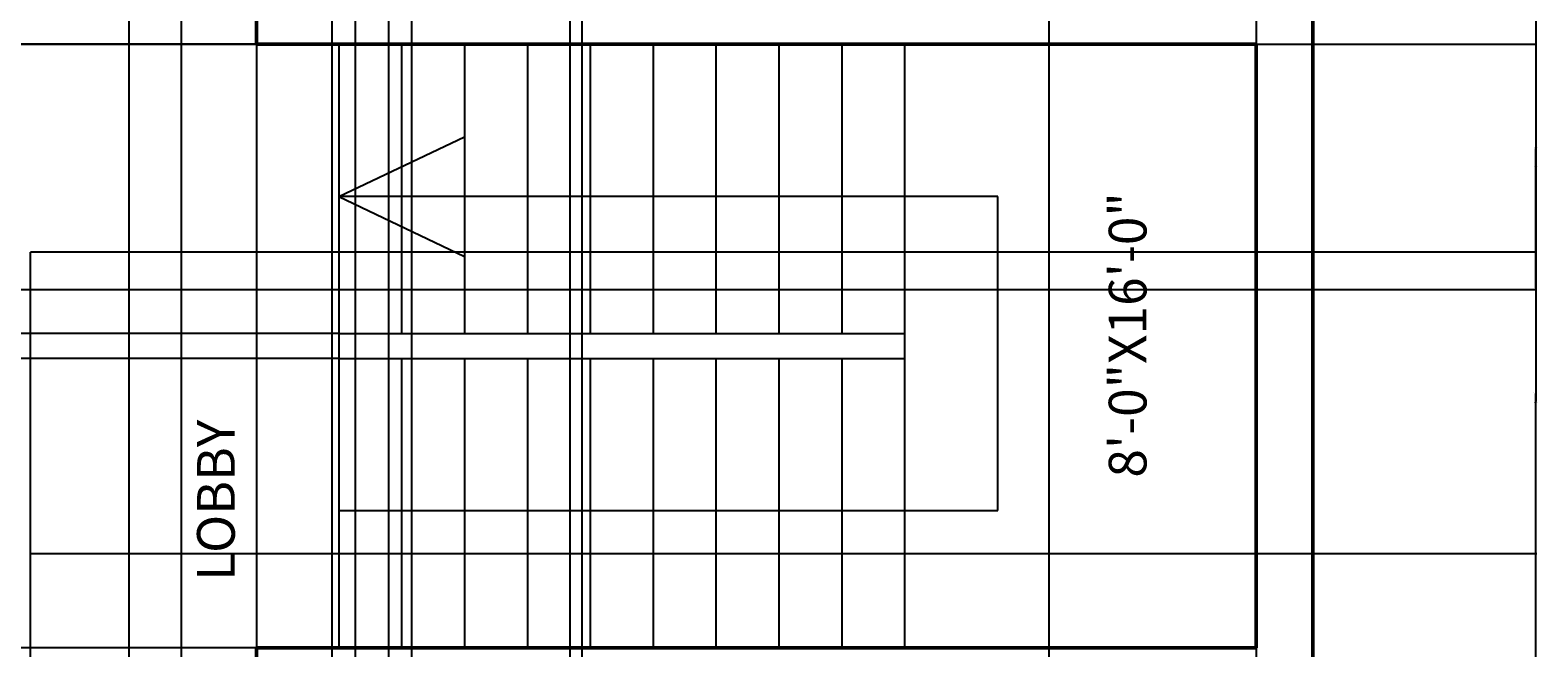
# Model space of a CAD drawing. Units: inches. Extents: x 3 to 576, y -689 to 51.
# Tile 13 of 21: x 336 to 576, y -359 to -261. Entities that reach past the tile are written whole.
import ezdxf

# ---------------------------------------------------------------- set-up
doc = ezdxf.new("R2010")
doc.units = ezdxf.units.IN
doc.header["$MEASUREMENT"] = 0
for name, color, linetype, lineweight in [('A-ANNO-DIMS', 2, 'Continuous', 18), ('A-AREA-IDEN', 7, 'Continuous', 18), ('A-FLOR-STRS', 7, 'Continuous', 25), ('A-WALL', 7, 'Continuous', 50)]:
    doc.layers.add(name, color=color, linetype=linetype, lineweight=lineweight)
doc.styles.get("Standard").update_dxf_attribs({"font": 'arial.ttf'})
doc.dimstyles.get("Standard").update_dxf_attribs({"dimtxt": 0.18, "dimasz": 0.18, "dimexe": 0.18, "dimexo": 0.0625, "dimgap": 0.09, "dimtad": 0, "dimtih": 1, "dimtoh": 1, "dimdec": 0, "dimzin": 0, "dimdsep": 46, "dimlunit": 3, "dimtxsty": 'Standard', "dimcen": 0.09, "dimadec": 0, "dimazin": 0, "dimtfac": 1, "dimtdec": 0, "dimtofl": 0, "dimtmove": 0, "dimatfit": 3, "dimfxl": 1, "dimtolj": 1, "dimtzin": 0, "dimarcsym": 0})

# ---------------------------------------------------------------- blocks, each defined once
blk = doc.blocks.new('*D39')
at = {"layer": 'A-ANNO-DIMS', "color": 0, "lineweight": -2, "transparency": 16777216}
for p, q in [((540.36, 15.69), (575.92, 15.69)), ((575.74, 15.51), (575.74, -318.63)), ((575.74, -653.13), (575.74, -318.99)), ((540.36, -653.31), (575.92, -653.31))]:
    blk.add_line(p, q, dxfattribs=at)
at = {"layer": 'A-ANNO-DIMS', "color": 0, "transparency": 16777216}
for points in [[(575.71, 15.51), (575.77, 15.51), (575.74, 15.69)], [(575.71, -653.13), (575.77, -653.13), (575.74, -653.31)]]:
    blk.add_solid(points, dxfattribs=at)
at = {"layer": 'Defpoints', "color": 0, "transparency": 16777216}
for p in [(540.29, 15.69), (540.29, -653.31), (575.74, -653.31)]:
    blk.add_point(p, dxfattribs=at)
at = {"layer": 'A-ANNO-DIMS', "color": 0, "transparency": 16777216, "insert": (575.74, -318.81), "char_height": 0.18, "attachment_point": 5}
blk.add_mtext('\\A1;55\'-9"', dxfattribs=at)
blk = doc.blocks.new('*D63')
at = {"layer": 'A-ANNO-DIMS', "color": 0, "lineweight": -2, "transparency": 16777216}
for p, q in [((47.36, -263.31), (575.92, -263.31)), ((575.74, -263.49), (575.74, -282.63)), ((575.74, -302.13), (575.74, -282.99)), ((47.36, -302.31), (575.92, -302.31))]:
    blk.add_line(p, q, dxfattribs=at)
at = {"layer": 'A-ANNO-DIMS', "color": 0, "transparency": 16777216}
for points in [[(575.71, -263.49), (575.77, -263.49), (575.74, -263.31)], [(575.71, -302.13), (575.77, -302.13), (575.74, -302.31)]]:
    blk.add_solid(points, dxfattribs=at)
at = {"layer": 'Defpoints', "color": 0, "transparency": 16777216}
for p in [(47.29, -263.31), (47.29, -302.31), (575.74, -302.31)]:
    blk.add_point(p, dxfattribs=at)
at = {"layer": 'A-ANNO-DIMS', "color": 0, "transparency": 16777216, "insert": (575.74, -282.81), "char_height": 0.18, "attachment_point": 5}
blk.add_mtext('\\A1;3\'-3"', dxfattribs=at)
blk = doc.blocks.new('*D68')
at = {"layer": 'A-ANNO-DIMS', "color": 0, "lineweight": -2, "transparency": 16777216}
for p, q in [((531.23, -254.31), (2.66, -254.31)), ((2.84, -254.49), (2.84, -258.63)), ((2.84, -263.13), (2.84, -258.99)), ((531.23, -263.31), (2.66, -263.31))]:
    blk.add_line(p, q, dxfattribs=at)
at = {"layer": 'A-ANNO-DIMS', "color": 0, "transparency": 16777216}
for points in [[(2.81, -254.49), (2.87, -254.49), (2.84, -254.31)], [(2.81, -263.13), (2.87, -263.13), (2.84, -263.31)]]:
    blk.add_solid(points, dxfattribs=at)
at = {"layer": 'Defpoints', "color": 0, "transparency": 16777216}
for p in [(531.29, -254.31), (2.84, -263.31), (531.29, -263.31)]:
    blk.add_point(p, dxfattribs=at)
at = {"layer": 'A-ANNO-DIMS', "color": 0, "transparency": 16777216, "insert": (2.84, -258.81), "char_height": 0.18, "attachment_point": 5}
blk.add_mtext('\\A1;0\'-9"', dxfattribs=at)
blk = doc.blocks.new('*D69')
at = {"layer": 'A-ANNO-DIMS', "color": 0, "lineweight": -2, "transparency": 16777216}
for p, q in [((531.23, -263.31), (2.66, -263.31)), ((2.84, -263.49), (2.84, -311.13)), ((2.84, -359.13), (2.84, -311.49)), ((531.23, -359.31), (2.66, -359.31))]:
    blk.add_line(p, q, dxfattribs=at)
at = {"layer": 'A-ANNO-DIMS', "color": 0, "transparency": 16777216}
for points in [[(2.81, -263.49), (2.87, -263.49), (2.84, -263.31)], [(2.81, -359.13), (2.87, -359.13), (2.84, -359.31)]]:
    blk.add_solid(points, dxfattribs=at)
at = {"layer": 'Defpoints', "color": 0, "transparency": 16777216}
for p in [(531.29, -263.31), (2.84, -359.31), (531.29, -359.31)]:
    blk.add_point(p, dxfattribs=at)
at = {"layer": 'A-ANNO-DIMS', "color": 0, "transparency": 16777216, "insert": (2.84, -311.31), "char_height": 0.18, "attachment_point": 5}
blk.add_mtext('\\A1;8\'-0"', dxfattribs=at)
blk = doc.blocks.new('*D76')
at = {"layer": 'A-ANNO-DIMS', "color": 0, "lineweight": -2, "transparency": 16777216}
for p, q in [((372.29, -263.37), (372.29, -688.94)), ((336.29, -296.37), (336.29, -688.94)), ((336.47, -688.76), (353.96, -688.76)), ((372.11, -688.76), (354.62, -688.76))]:
    blk.add_line(p, q, dxfattribs=at)
at = {"layer": 'A-ANNO-DIMS', "color": 0, "transparency": 16777216}
for points in [[(336.47, -688.73), (336.47, -688.79), (336.29, -688.76)], [(372.11, -688.73), (372.11, -688.79), (372.29, -688.76)]]:
    blk.add_solid(points, dxfattribs=at)
at = {"layer": 'Defpoints', "color": 0, "transparency": 16777216}
for p in [(372.29, -263.31), (336.29, -296.31), (372.29, -688.76)]:
    blk.add_point(p, dxfattribs=at)
at = {"layer": 'A-ANNO-DIMS', "color": 0, "transparency": 16777216, "insert": (354.29, -688.76), "char_height": 0.18, "attachment_point": 5}
blk.add_mtext('\\A1;3\'-0"', dxfattribs=at)
blk = doc.blocks.new('*D77')
at = {"layer": 'A-ANNO-DIMS', "color": 0, "lineweight": -2, "transparency": 16777216}
for p, q in [((372.29, -263.37), (372.29, -688.94)), ((531.29, -263.37), (531.29, -688.94)), ((372.47, -688.76), (451.4, -688.76)), ((531.11, -688.76), (452.18, -688.76))]:
    blk.add_line(p, q, dxfattribs=at)
at = {"layer": 'A-ANNO-DIMS', "color": 0, "transparency": 16777216}
for points in [[(372.47, -688.73), (372.47, -688.79), (372.29, -688.76)], [(531.11, -688.73), (531.11, -688.79), (531.29, -688.76)]]:
    blk.add_solid(points, dxfattribs=at)
at = {"layer": 'Defpoints', "color": 0, "transparency": 16777216}
for p in [(372.29, -263.31), (531.29, -263.31), (531.29, -688.76)]:
    blk.add_point(p, dxfattribs=at)
at = {"layer": 'A-ANNO-DIMS', "color": 0, "transparency": 16777216, "insert": (451.79, -688.76), "char_height": 0.18, "attachment_point": 5}
blk.add_mtext('\\A1;13\'-3"', dxfattribs=at)
blk = doc.blocks.new('*D78')
at = {"layer": 'A-ANNO-DIMS', "color": 0, "lineweight": -2, "transparency": 16777216}
for p, q in [((336.36, -263.31), (575.92, -263.31)), ((575.74, -263.49), (575.74, -279.63)), ((575.74, -296.13), (575.74, -279.99)), ((336.36, -296.31), (575.92, -296.31))]:
    blk.add_line(p, q, dxfattribs=at)
at = {"layer": 'A-ANNO-DIMS', "color": 0, "transparency": 16777216}
for points in [[(575.71, -263.49), (575.77, -263.49), (575.74, -263.31)], [(575.71, -296.13), (575.77, -296.13), (575.74, -296.31)]]:
    blk.add_solid(points, dxfattribs=at)
at = {"layer": 'Defpoints', "color": 0, "transparency": 16777216}
for p in [(336.29, -263.31), (336.29, -296.31), (575.74, -296.31)]:
    blk.add_point(p, dxfattribs=at)
at = {"layer": 'A-ANNO-DIMS', "color": 0, "transparency": 16777216, "insert": (575.74, -279.81), "char_height": 0.18, "attachment_point": 5}
blk.add_mtext('\\A1;2\'-9"', dxfattribs=at)
blk = doc.blocks.new('*D79')
at = {"layer": 'A-ANNO-DIMS', "color": 0, "lineweight": -2, "transparency": 16777216}
for p, q in [((336.36, -296.31), (575.92, -296.31)), ((575.74, -296.49), (575.74, -320.13)), ((575.74, -344.13), (575.74, -320.49)), ((336.36, -344.31), (575.92, -344.31))]:
    blk.add_line(p, q, dxfattribs=at)
at = {"layer": 'A-ANNO-DIMS', "color": 0, "transparency": 16777216}
for points in [[(575.71, -296.49), (575.77, -296.49), (575.74, -296.31)], [(575.71, -344.13), (575.77, -344.13), (575.74, -344.31)]]:
    blk.add_solid(points, dxfattribs=at)
at = {"layer": 'Defpoints', "color": 0, "transparency": 16777216}
for p in [(336.29, -296.31), (336.29, -344.31), (575.74, -344.31)]:
    blk.add_point(p, dxfattribs=at)
at = {"layer": 'A-ANNO-DIMS', "color": 0, "transparency": 16777216, "insert": (575.74, -320.31), "char_height": 0.18, "attachment_point": 5}
blk.add_mtext('\\A1;4\'-0"', dxfattribs=at)
blk = doc.blocks.new('*D84')
at = {"layer": 'A-ANNO-DIMS', "color": 0, "lineweight": -2, "transparency": 16777216}
for p, q in [((385.3, -263.31), (2.66, -263.31)), ((2.84, -263.49), (2.84, -286.13)), ((2.84, -309.13), (2.84, -286.49)), ((385.3, -309.31), (2.66, -309.31))]:
    blk.add_line(p, q, dxfattribs=at)
at = {"layer": 'A-ANNO-DIMS', "color": 0, "transparency": 16777216}
for points in [[(2.81, -263.49), (2.87, -263.49), (2.84, -263.31)], [(2.81, -309.13), (2.87, -309.13), (2.84, -309.31)]]:
    blk.add_solid(points, dxfattribs=at)
at = {"layer": 'Defpoints', "color": 0, "transparency": 16777216}
for p in [(385.37, -263.31), (2.84, -309.31), (385.37, -309.31)]:
    blk.add_point(p, dxfattribs=at)
at = {"layer": 'A-ANNO-DIMS', "color": 0, "transparency": 16777216, "insert": (2.84, -286.31), "char_height": 0.18, "attachment_point": 5}
blk.add_mtext('\\A1;3\'-10"', dxfattribs=at)
blk = doc.blocks.new('*D85')
at = {"layer": 'A-ANNO-DIMS', "color": 0, "lineweight": -2, "transparency": 16777216}
for p, q in [((385.3, -313.31), (2.66, -313.31)), ((2.84, -313.49), (2.84, -336.13)), ((2.84, -359.13), (2.84, -336.49)), ((385.3, -359.31), (2.66, -359.31))]:
    blk.add_line(p, q, dxfattribs=at)
at = {"layer": 'A-ANNO-DIMS', "color": 0, "transparency": 16777216}
for points in [[(2.81, -313.49), (2.87, -313.49), (2.84, -313.31)], [(2.81, -359.13), (2.87, -359.13), (2.84, -359.31)]]:
    blk.add_solid(points, dxfattribs=at)
at = {"layer": 'Defpoints', "color": 0, "transparency": 16777216}
for p in [(385.37, -313.31), (2.84, -359.31), (385.37, -359.31)]:
    blk.add_point(p, dxfattribs=at)
at = {"layer": 'A-ANNO-DIMS', "color": 0, "transparency": 16777216, "insert": (2.84, -336.31), "char_height": 0.18, "attachment_point": 5}
blk.add_mtext('\\A1;3\'-10"', dxfattribs=at)
blk = doc.blocks.new('*D94')
at = {"layer": 'A-ANNO-DIMS', "color": 0, "lineweight": -2, "transparency": 16777216}
for p, q in [((393.29, -136.9), (393.29, -688.94)), ((422.14, -136.9), (422.14, -688.94)), ((393.47, -688.76), (407.39, -688.76)), ((421.96, -688.76), (408.05, -688.76))]:
    blk.add_line(p, q, dxfattribs=at)
at = {"layer": 'A-ANNO-DIMS', "color": 0, "transparency": 16777216}
for points in [[(393.47, -688.73), (393.47, -688.79), (393.29, -688.76)], [(421.96, -688.73), (421.96, -688.79), (422.14, -688.76)]]:
    blk.add_solid(points, dxfattribs=at)
at = {"layer": 'Defpoints', "color": 0, "transparency": 16777216}
for p in [(393.29, -136.84), (422.14, -136.84), (422.14, -688.76)]:
    blk.add_point(p, dxfattribs=at)
at = {"layer": 'A-ANNO-DIMS', "color": 0, "transparency": 16777216, "insert": (407.72, -688.76), "char_height": 0.18, "attachment_point": 5}
blk.add_mtext('\\A1;2\'-5"', dxfattribs=at)
blk = doc.blocks.new('*D96')
at = {"layer": 'A-ANNO-DIMS', "color": 0, "lineweight": -2, "transparency": 16777216}
for p, q in [((397.02, -506.04), (397.02, 51.32)), ((397.2, 51.14), (410.22, 51.14)), ((423.91, 51.14), (410.89, 51.14)), ((424.09, -506.04), (424.09, 51.32))]:
    blk.add_line(p, q, dxfattribs=at)
at = {"layer": 'A-ANNO-DIMS', "color": 0, "transparency": 16777216}
for points in [[(397.2, 51.17), (397.2, 51.11), (397.02, 51.14)], [(423.91, 51.17), (423.91, 51.11), (424.09, 51.14)]]:
    blk.add_solid(points, dxfattribs=at)
at = {"layer": 'Defpoints', "color": 0, "transparency": 16777216}
for p in [(424.09, 51.14), (397.02, -506.1), (424.09, -506.1)]:
    blk.add_point(p, dxfattribs=at)
at = {"layer": 'A-ANNO-DIMS', "color": 0, "transparency": 16777216, "insert": (410.56, 51.14), "char_height": 0.18, "attachment_point": 5}
blk.add_mtext('\\A1;2\'-3"', dxfattribs=at)
blk = doc.blocks.new('*D103')
at = {"layer": 'A-ANNO-DIMS', "color": 0, "lineweight": -2, "transparency": 16777216}
for p, q in [((498.29, -50.37), (498.29, -688.94)), ((531.29, -50.37), (531.29, -688.94)), ((498.47, -688.76), (514.46, -688.76)), ((531.11, -688.76), (515.12, -688.76))]:
    blk.add_line(p, q, dxfattribs=at)
at = {"layer": 'A-ANNO-DIMS', "color": 0, "transparency": 16777216}
for points in [[(498.47, -688.73), (498.47, -688.79), (498.29, -688.76)], [(531.11, -688.73), (531.11, -688.79), (531.29, -688.76)]]:
    blk.add_solid(points, dxfattribs=at)
at = {"layer": 'Defpoints', "color": 0, "transparency": 16777216}
for p in [(498.29, -50.31), (531.29, -50.31), (531.29, -688.76)]:
    blk.add_point(p, dxfattribs=at)
at = {"layer": 'A-ANNO-DIMS', "color": 0, "transparency": 16777216, "insert": (514.79, -688.76), "char_height": 0.18, "attachment_point": 5}
blk.add_mtext('\\A1;2\'-9"', dxfattribs=at)
blk = doc.blocks.new('*D116')
at = {"layer": 'A-ANNO-DIMS', "color": 0, "lineweight": -2, "transparency": 16777216}
for p, q in [((360.29, -134.37), (360.29, -688.94)), ((384.29, -134.37), (384.29, -688.94)), ((360.47, -688.76), (371.96, -688.76)), ((384.11, -688.76), (372.62, -688.76))]:
    blk.add_line(p, q, dxfattribs=at)
at = {"layer": 'A-ANNO-DIMS', "color": 0, "transparency": 16777216}
for points in [[(360.47, -688.73), (360.47, -688.79), (360.29, -688.76)], [(384.11, -688.73), (384.11, -688.79), (384.29, -688.76)]]:
    blk.add_solid(points, dxfattribs=at)
at = {"layer": 'Defpoints', "color": 0, "transparency": 16777216}
for p in [(360.29, -134.31), (384.29, -134.31), (384.29, -688.76)]:
    blk.add_point(p, dxfattribs=at)
at = {"layer": 'A-ANNO-DIMS', "color": 0, "transparency": 16777216, "insert": (372.29, -688.76), "char_height": 0.18, "attachment_point": 5}
blk.add_mtext('\\A1;2\'-0"', dxfattribs=at)
blk = doc.blocks.new('*D118')
at = {"layer": 'A-ANNO-DIMS', "color": 0, "lineweight": -2, "transparency": 16777216}
for p, q in [((352.02, -506.25), (352.02, 51.32)), ((352.2, 51.14), (369.69, 51.14)), ((387.84, 51.14), (370.35, 51.14)), ((388.02, -506.25), (388.02, 51.32))]:
    blk.add_line(p, q, dxfattribs=at)
at = {"layer": 'A-ANNO-DIMS', "color": 0, "transparency": 16777216}
for points in [[(352.2, 51.17), (352.2, 51.11), (352.02, 51.14)], [(387.84, 51.17), (387.84, 51.11), (388.02, 51.14)]]:
    blk.add_solid(points, dxfattribs=at)
at = {"layer": 'Defpoints', "color": 0, "transparency": 16777216}
for p in [(388.02, 51.14), (352.02, -506.31), (388.02, -506.31)]:
    blk.add_point(p, dxfattribs=at)
at = {"layer": 'A-ANNO-DIMS', "color": 0, "transparency": 16777216, "insert": (370.02, 51.14), "char_height": 0.18, "attachment_point": 5}
blk.add_mtext('\\A1;3\'-0"', dxfattribs=at)

msp = doc.modelspace()

# ---------------------------------------------------------------- linework, layer by layer
at = {"layer": 'A-FLOR-STRS'}
for p, q in [((385.37, -263.31), (385.37, -359.31)), ((395.37, -263.31), (395.37, -309.31)), ((405.37, -263.31), (405.37, -309.31)), ((415.37, -263.31), (415.37, -309.31)), ((425.37, -263.31), (425.37, -309.31)), ((435.37, -263.31), (435.37, -309.31)), ((445.37, -263.31), (445.37, -309.31)), ((455.37, -263.31), (455.37, -309.31)), ((465.37, -263.31), (465.37, -309.31)), ((475.37, -263.31), (475.37, -359.31)), ((385.37, -287.55), (405.37, -278.02)), ((490.22, -287.55), (385.37, -287.55)), ((385.37, -287.55), (405.37, -297.09)), ((490.22, -337.45), (490.22, -287.55)), ((385.37, -309.31), (475.37, -309.31)), ((385.37, -313.31), (475.37, -313.31)), ((395.37, -313.31), (395.37, -359.31)), ((405.37, -313.31), (405.37, -359.31)), ((415.37, -313.31), (415.37, -359.31)), ((425.37, -313.31), (425.37, -359.31)), ((435.37, -313.31), (435.37, -359.31)), ((445.37, -313.31), (445.37, -359.31)), ((455.37, -313.31), (455.37, -359.31)), ((465.37, -313.31), (465.37, -359.31)), ((385.37, -337.45), (490.22, -337.45))]:
    msp.add_line(p, q, dxfattribs=at)
at = {"layer": 'A-WALL'}
for p, q in [((540.29, 15.69), (540.29, -653.31)), ((372.29, -254.31), (372.29, -263.31)), ((372.29, -263.31), (531.29, -263.31)), ((531.29, -263.31), (531.29, -359.31)), ((372.29, -359.31), (531.29, -359.31)), ((372.29, -368.31), (372.29, -359.31))]:
    msp.add_line(p, q, dxfattribs=at)

# ---------------------------------------------------------------- texts
at = {"layer": 'A-AREA-IDEN', "insert": (507.84, -332.24), "char_height": 6, "attachment_point": 1, "rotation": 90}
msp.add_mtext_dynamic_manual_height_columns('8\'-0"X16\'-0"', width=6, gutter_width=1, heights=[0], dxfattribs=at)
at = {"layer": 'A-AREA-IDEN', "insert": (362.84, -348.66), "char_height": 6, "attachment_point": 1, "rotation": 90}
msp.add_mtext('LOBBY', dxfattribs=at)

# ---------------------------------------------------------------- dimensions: what is measured, and where the dimension line sits
at = {"layer": 'A-ANNO-DIMS'}
for base, p1, p2, picture, middle in [((388.02, 51.14), (352.02, -506.31), (388.02, -506.31), '*D118', (370.02, 51.14)), ((424.09, 51.14), (397.02, -506.1), (424.09, -506.1), '*D96', (410.56, 51.14)), ((531.29, -688.76), (498.29, -50.31), (531.29, -50.31), '*D103', (514.79, -688.76)), ((384.29, -688.76), (360.29, -134.31), (384.29, -134.31), '*D116', (372.29, -688.76)), ((422.1383, -688.7597), (393.294, -136.8425), (422.1383, -136.8425), '*D94', (407.7162, -688.7597)), ((372.29, -688.76), (336.29, -296.31), (372.29, -263.31), '*D76', (354.29, -688.76)), ((531.29, -688.76), (372.29, -263.31), (531.29, -263.31), '*D77', (451.79, -688.76))]:
    dim = msp.add_linear_dim(base=base, p1=p1, p2=p2, dimstyle='Standard', override={"dimdec": 1, "dimlfac": 1, "dimrnd": 0, "dimzin": 1, "dimdsep": 46, "dimlunit": 4, "dimfrac": 2}, dxfattribs=at)
    dim.commit()
    dim.dimension.update_dxf_attribs({"geometry": picture, "text_midpoint": middle})
for base, p1, p2, picture, middle in [((575.74, -653.31), (540.29, 15.69), (540.29, -653.31), '*D39', (575.74, -318.81)), ((2.84, -263.31), (531.29, -254.31), (531.29, -263.31), '*D68', (2.84, -258.81)), ((2.84, -309.31), (385.37, -263.31), (385.37, -309.31), '*D84', (2.84, -286.31)), ((2.84, -359.31), (531.29, -263.31), (531.29, -359.31), '*D69', (2.84, -311.31)), ((575.74, -302.31), (47.29, -263.31), (47.29, -302.31), '*D63', (575.74, -282.81)), ((575.74, -296.31), (336.29, -263.31), (336.29, -296.31), '*D78', (575.74, -279.81)), ((575.74, -344.31), (336.29, -296.31), (336.29, -344.31), '*D79', (575.74, -320.31)), ((2.84, -359.31), (385.37, -313.31), (385.37, -359.31), '*D85', (2.84, -336.31))]:
    dim = msp.add_linear_dim(base=base, p1=p1, p2=p2, angle=90, dimstyle='Standard', override={"dimdec": 1, "dimlfac": 1, "dimrnd": 0, "dimzin": 1, "dimdsep": 46, "dimlunit": 4, "dimfrac": 2}, dxfattribs=at)
    dim.commit()
    dim.dimension.update_dxf_attribs({"geometry": picture, "text_midpoint": middle})

doc.saveas('drawing.dxf')
